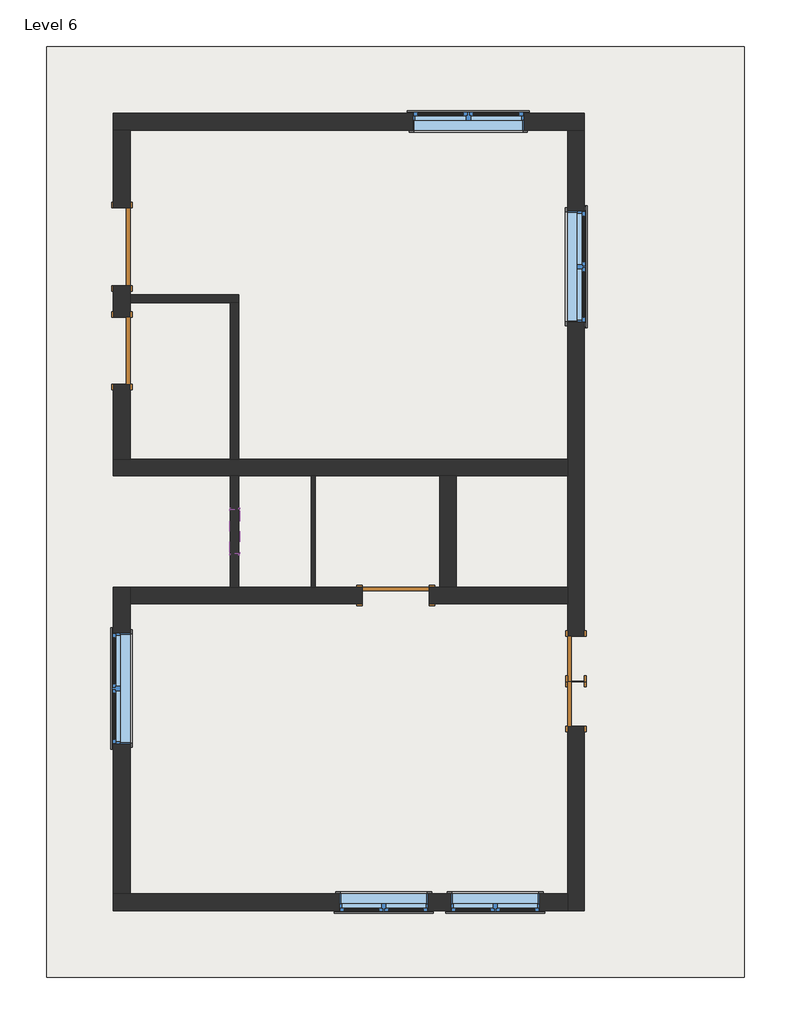
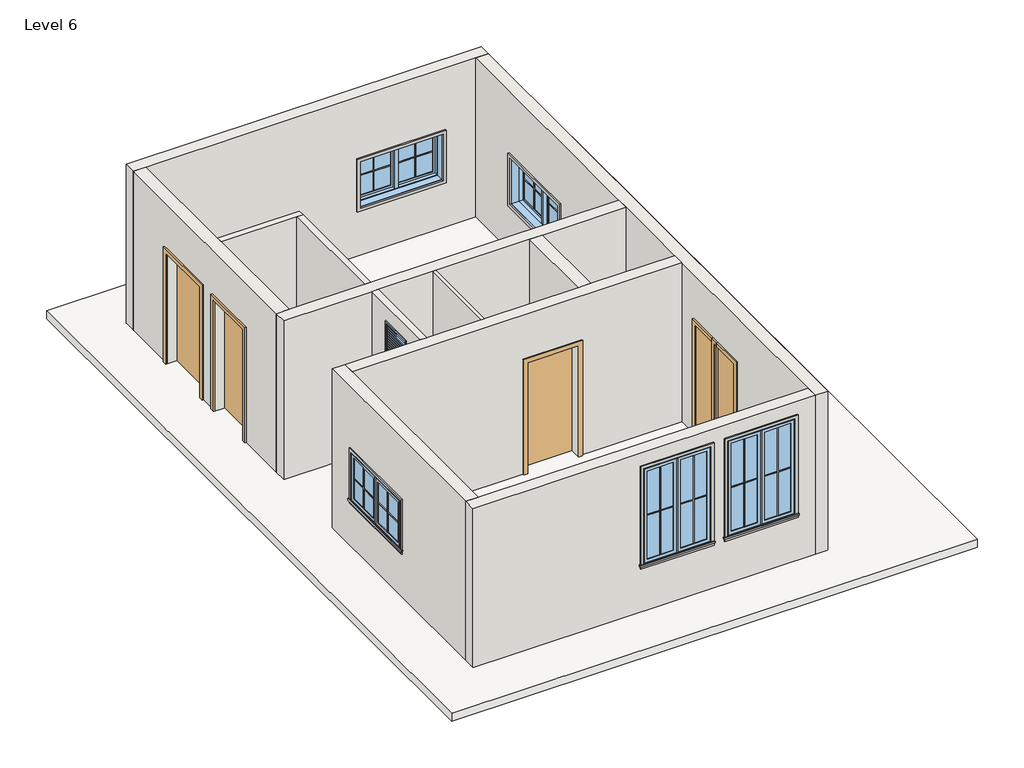
# One storey, incomplete: 20 proxies, 12 walls, 6 windows, 5 doors, 1 roof.
"""IFC4 building model written with IfcOpenShell, lengths in millimetres."""

from ifc_helpers import new_model, si_unit, frame, origin, place, context, project, spatial, polyline, outline, extrude, faceted_brep, transform, mapped, element, save
from components import muntin_pattern_2x2_muntin_pattern_2x2_9352d081, muntin_pattern_2x2_muntin_pattern_2x2_5c2cbe28, muntin_pattern_2x2_muntin_pattern_2x2_2b4d9f72, muntin_pattern_2x2_muntin_pattern_2x2_ef995ed3, trim_window_exterior_flat_with_sill_979bde60, trim_window_exterior_flat_with_sill_b7e4d11c, trim_window_interior_flat_picture_frame_7883d11b, trim_window_interior_flat_picture_frame_936b8d2a, single_flush_door_2_0d3b4037, single_flush_door_2_4a3212df, door_a90ba1ad, door_0ca8825f, door_9d399b00, window_casement_double_c1d95f0f, window_casement_double_wall_4_6ca1769e, window_d39e7ecb

model = new_model("IFC4")

# Units and contexts
model_context = context("Model", 3, world=origin())
ifc_project = project(units=[si_unit("LENGTHUNIT", "METRE", prefix="MILLI")], contexts=[model_context])

# Site, building, storey
site = spatial("IfcSite", under=ifc_project)
building = spatial("IfcBuilding", under=site)
storey = spatial("IfcBuildingStorey", under=building, Name="Level 6", Elevation=12801.6)

# Proxies
placement = place(None, origin())
muntin_pattern_2x2_muntin_pattern_2x2_shape = muntin_pattern_2x2_muntin_pattern_2x2_9352d081(model_context)
element("IfcBuildingElementProxy", 1, Name="Muntin Pattern_2x2 : Muntin Pattern_2x2", ObjectType="Muntin Pattern_2x2 : Muntin Pattern_2x2", at=placement, inside=storey, context=model_context, shape_type="MappedRepresentation", body=[
    mapped(muntin_pattern_2x2_muntin_pattern_2x2_shape, transform((-4785.3510342, -2707.8617544, 13785.85), x_axis=(0.0, 1.0, 0.0), y_axis=(-1.0, 0.0, 0.0), z_axis=(0.0, 0.0, 1.0))),
])
element("IfcBuildingElementProxy", 2, Name="Muntin Pattern_2x2 : Muntin Pattern_2x2", ObjectType="Muntin Pattern_2x2 : Muntin Pattern_2x2", at=placement, inside=storey, context=model_context, shape_type="MappedRepresentation", body=[
    mapped(muntin_pattern_2x2_muntin_pattern_2x2_shape, transform((1634.4989658, 3816.7632456, 13785.85), x_axis=(0.0, -1.0, 0.0), y_axis=(1.0, 0.0, 0.0), z_axis=(0.0, 0.0, 1.0))),
])
element("IfcBuildingElementProxy", 3, Name="Muntin Pattern_2x2 : Muntin Pattern_2x2", ObjectType="Muntin Pattern_2x2 : Muntin Pattern_2x2", at=placement, inside=storey, context=model_context, shape_type="MappedRepresentation", body=[
    mapped(muntin_pattern_2x2_muntin_pattern_2x2_shape, transform((-322.8885342, 5523.3257456, 13785.85), x_axis=(1.0, 0.0, 0.0), y_axis=(0.0, 1.0, 0.0), z_axis=(0.0, 0.0, 1.0))),
])
muntin_pattern_2x2_muntin_pattern_2x2_2_shape = muntin_pattern_2x2_muntin_pattern_2x2_5c2cbe28(model_context)
element("IfcBuildingElementProxy", 4, Name="Muntin Pattern_2x2 : Muntin Pattern_2x2", ObjectType="Muntin Pattern_2x2 : Muntin Pattern_2x2", at=placement, inside=storey, context=model_context, shape_type="MappedRepresentation", body=[
    mapped(muntin_pattern_2x2_muntin_pattern_2x2_2_shape, transform((-4785.3510342, -1949.0367544, 13785.85), x_axis=(0.0, -1.0, 0.0), y_axis=(1.0, 0.0, 0.0), z_axis=(0.0, 0.0, 1.0))),
])
element("IfcBuildingElementProxy", 5, Name="Muntin Pattern_2x2 : Muntin Pattern_2x2", ObjectType="Muntin Pattern_2x2 : Muntin Pattern_2x2", at=placement, inside=storey, context=model_context, shape_type="MappedRepresentation", body=[
    mapped(muntin_pattern_2x2_muntin_pattern_2x2_2_shape, transform((1634.4989658, 3057.9382456, 13785.85), x_axis=(0.0, 1.0, 0.0), y_axis=(-1.0, 0.0, 0.0), z_axis=(0.0, 0.0, 1.0))),
])
element("IfcBuildingElementProxy", 6, Name="Muntin Pattern_2x2 : Muntin Pattern_2x2", ObjectType="Muntin Pattern_2x2 : Muntin Pattern_2x2", at=placement, inside=storey, context=model_context, shape_type="MappedRepresentation", body=[
    mapped(muntin_pattern_2x2_muntin_pattern_2x2_2_shape, transform((435.9364658, 5523.3257456, 13785.85), x_axis=(-1.0, 0.0, 0.0), y_axis=(0.0, -1.0, 0.0), z_axis=(0.0, 0.0, 1.0))),
])
muntin_pattern_2x2_muntin_pattern_2x2_3_shape = muntin_pattern_2x2_muntin_pattern_2x2_2b4d9f72(model_context)
element("IfcBuildingElementProxy", 7, Name="Muntin Pattern_2x2 : Muntin Pattern_2x2", ObjectType="Muntin Pattern_2x2 : Muntin Pattern_2x2", at=placement, inside=storey, context=model_context, shape_type="MappedRepresentation", body=[
    mapped(muntin_pattern_2x2_muntin_pattern_2x2_3_shape, transform((-795.9635342, -5354.2242544, 13785.85), x_axis=(-1.0, 0.0, 0.0), y_axis=(0.0, -1.0, 0.0), z_axis=(0.0, 0.0, 1.0))),
])
element("IfcBuildingElementProxy", 8, Name="Muntin Pattern_2x2 : Muntin Pattern_2x2", ObjectType="Muntin Pattern_2x2 : Muntin Pattern_2x2", at=placement, inside=storey, context=model_context, shape_type="MappedRepresentation", body=[
    mapped(muntin_pattern_2x2_muntin_pattern_2x2_3_shape, transform((728.0364658, -5354.2242544, 13785.85), x_axis=(-1.0, 0.0, 0.0), y_axis=(0.0, -1.0, 0.0), z_axis=(0.0, 0.0, 1.0))),
])
muntin_pattern_2x2_muntin_pattern_2x2_4_shape = muntin_pattern_2x2_muntin_pattern_2x2_ef995ed3(model_context)
element("IfcBuildingElementProxy", 9, Name="Muntin Pattern_2x2 : Muntin Pattern_2x2", ObjectType="Muntin Pattern_2x2 : Muntin Pattern_2x2", at=placement, inside=storey, context=model_context, shape_type="MappedRepresentation", body=[
    mapped(muntin_pattern_2x2_muntin_pattern_2x2_4_shape, transform((-1402.3885342, -5354.2242544, 13785.85), x_axis=(1.0, 0.0, 0.0), y_axis=(0.0, 1.0, 0.0), z_axis=(0.0, 0.0, 1.0))),
])
element("IfcBuildingElementProxy", 10, Name="Muntin Pattern_2x2 : Muntin Pattern_2x2", ObjectType="Muntin Pattern_2x2 : Muntin Pattern_2x2", at=placement, inside=storey, context=model_context, shape_type="MappedRepresentation", body=[
    mapped(muntin_pattern_2x2_muntin_pattern_2x2_4_shape, transform((121.6114658, -5354.2242544, 13785.85), x_axis=(1.0, 0.0, 0.0), y_axis=(0.0, 1.0, 0.0), z_axis=(0.0, 0.0, 1.0))),
])
trim_window_exterior_flat_with_sill_shape = trim_window_exterior_flat_with_sill_979bde60(model_context)
element("IfcBuildingElementProxy", 11, Name="Trim-Window-Exterior-Flat : with Sill", ObjectType="Trim-Window-Exterior-Flat : with Sill", at=placement, inside=storey, context=model_context, shape_type="MappedRepresentation", body=[
    mapped(trim_window_exterior_flat_with_sill_shape, transform((-4794.8760342, -2328.4492544, 14630.4), x_axis=(0.0, -1.0, 0.0), y_axis=(0.0, 0.0, 1.0), z_axis=(-1.0, 0.0, 0.0))),
])
element("IfcBuildingElementProxy", 12, Name="Trim-Window-Exterior-Flat : with Sill", ObjectType="Trim-Window-Exterior-Flat : with Sill", at=placement, inside=storey, context=model_context, shape_type="MappedRepresentation", body=[
    mapped(trim_window_exterior_flat_with_sill_shape, transform((1644.0239658, 3437.3507456, 14630.4), x_axis=(0.0, 1.0, 0.0), y_axis=(0.0, 0.0, 1.0), z_axis=(1.0, 0.0, 0.0))),
])
element("IfcBuildingElementProxy", 13, Name="Trim-Window-Exterior-Flat : with Sill", ObjectType="Trim-Window-Exterior-Flat : with Sill", at=placement, inside=storey, context=model_context, shape_type="MappedRepresentation", body=[
    mapped(trim_window_exterior_flat_with_sill_shape, transform((56.5239658, 5532.8507456, 14630.4), x_axis=(-1.0, 0.0, 0.0), y_axis=(0.0, 0.0, 1.0), z_axis=(0.0, 1.0, 0.0))),
])
trim_window_exterior_flat_with_sill_2_shape = trim_window_exterior_flat_with_sill_b7e4d11c(model_context)
element("IfcBuildingElementProxy", 14, Name="Trim-Window-Exterior-Flat : with Sill", ObjectType="Trim-Window-Exterior-Flat : with Sill", at=placement, inside=storey, context=model_context, shape_type="MappedRepresentation", body=[
    mapped(trim_window_exterior_flat_with_sill_2_shape, transform((-1099.1760342, -5363.7492544, 15544.8), x_axis=(1.0, 0.0, 0.0), y_axis=(0.0, 0.0, 1.0), z_axis=(0.0, -1.0, 0.0))),
])
element("IfcBuildingElementProxy", 15, Name="Trim-Window-Exterior-Flat : with Sill", ObjectType="Trim-Window-Exterior-Flat : with Sill", at=placement, inside=storey, context=model_context, shape_type="MappedRepresentation", body=[
    mapped(trim_window_exterior_flat_with_sill_2_shape, transform((424.8239658, -5363.7492544, 15544.8), x_axis=(1.0, 0.0, 0.0), y_axis=(0.0, 0.0, 1.0), z_axis=(0.0, -1.0, 0.0))),
])
trim_window_interior_flat_picture_frame_shape = trim_window_interior_flat_picture_frame_7883d11b(model_context)
element("IfcBuildingElementProxy", 16, Name="Trim-Window-Interior-Flat : Picture Frame", ObjectType="Trim-Window-Interior-Flat : Picture Frame", at=placement, inside=storey, context=model_context, shape_type="MappedRepresentation", body=[
    mapped(trim_window_interior_flat_picture_frame_shape, transform((-4566.2760342, -2328.4492544, 14630.4), x_axis=(0.0, 1.0, 0.0), y_axis=(0.0, 0.0, 1.0), z_axis=(1.0, 0.0, 0.0))),
])
element("IfcBuildingElementProxy", 17, Name="Trim-Window-Interior-Flat : Picture Frame", ObjectType="Trim-Window-Interior-Flat : Picture Frame", at=placement, inside=storey, context=model_context, shape_type="MappedRepresentation", body=[
    mapped(trim_window_interior_flat_picture_frame_shape, transform((1415.4239658, 3437.3507456, 14630.4), x_axis=(0.0, -1.0, 0.0), y_axis=(0.0, 0.0, 1.0), z_axis=(-1.0, 0.0, 0.0))),
])
element("IfcBuildingElementProxy", 18, Name="Trim-Window-Interior-Flat : Picture Frame", ObjectType="Trim-Window-Interior-Flat : Picture Frame", at=placement, inside=storey, context=model_context, shape_type="MappedRepresentation", body=[
    mapped(trim_window_interior_flat_picture_frame_shape, transform((56.5239658, 5304.2507456, 14630.4), x_axis=(1.0, 0.0, 0.0), y_axis=(0.0, 0.0, 1.0), z_axis=(0.0, -1.0, 0.0))),
])
trim_window_interior_flat_picture_frame_2_shape = trim_window_interior_flat_picture_frame_936b8d2a(model_context)
element("IfcBuildingElementProxy", 19, Name="Trim-Window-Interior-Flat : Picture Frame", ObjectType="Trim-Window-Interior-Flat : Picture Frame", at=placement, inside=storey, context=model_context, shape_type="MappedRepresentation", body=[
    mapped(trim_window_interior_flat_picture_frame_2_shape, transform((-1099.1760342, -5135.1492544, 15544.8), x_axis=(-1.0, 0.0, 0.0), y_axis=(0.0, 0.0, 1.0), z_axis=(0.0, 1.0, 0.0))),
])
element("IfcBuildingElementProxy", 20, Name="Trim-Window-Interior-Flat : Picture Frame", ObjectType="Trim-Window-Interior-Flat : Picture Frame", at=placement, inside=storey, context=model_context, shape_type="MappedRepresentation", body=[
    mapped(trim_window_interior_flat_picture_frame_2_shape, transform((424.8239658, -5135.1492544, 15544.8), x_axis=(-1.0, 0.0, 0.0), y_axis=(0.0, 0.0, 1.0), z_axis=(0.0, 1.0, 0.0))),
])

# Doors
single_flush_door_2_shape = single_flush_door_2_0d3b4037(model_context)
element("IfcDoor", 21, ObjectType="Single-Flush : door 2'", at=placement, inside=storey, context=model_context, shape_type="MappedRepresentation", body=[
    mapped(single_flush_door_2_shape, transform((1529.7239658, -1922.0492544, 12801.6), x_axis=(0.0, 1.0, 0.0), y_axis=(-1.0, 0.0, 0.0), z_axis=(0.0, 0.0, 1.0))),
])
single_flush_door_2_2_shape = single_flush_door_2_4a3212df(model_context)
element("IfcDoor", 22, ObjectType="Single-Flush : door 2'", at=placement, inside=storey, context=model_context, shape_type="MappedRepresentation", body=[
    mapped(single_flush_door_2_2_shape, transform((1529.7239658, -2537.9992544, 12801.6), x_axis=(0.0, -1.0, 0.0), y_axis=(1.0, 0.0, 0.0), z_axis=(0.0, 0.0, 1.0))),
])
door_shape = door_a90ba1ad(model_context)
element("IfcDoor", 23, ObjectType="Single-Flush : door 2'6\"", at=placement, inside=storey, context=model_context, shape_type="MappedRepresentation", body=[
    mapped(door_shape, transform((-4680.5760342, 2288.0007456, 12801.6), x_axis=(0.0, 1.0, 0.0), y_axis=(-1.0, 0.0, 0.0), z_axis=(0.0, 0.0, 1.0))),
])
door_2_shape = door_0ca8825f(model_context)
element("IfcDoor", 24, ObjectType="Single-Flush : door 2'6\"", at=placement, inside=storey, context=model_context, shape_type="MappedRepresentation", body=[
    mapped(door_2_shape, transform((-934.0760342, -1058.4492544, 12801.6), x_axis=(1.0, 0.0, 0.0), y_axis=(0.0, 1.0, 0.0), z_axis=(0.0, 0.0, 1.0))),
])
door_3_shape = door_9d399b00(model_context)
element("IfcDoor", 25, ObjectType="Single-Flush : door 3'6\"", at=placement, inside=storey, context=model_context, shape_type="MappedRepresentation", body=[
    mapped(door_3_shape, transform((-4680.5760342, 3710.4007456, 12801.6), x_axis=(0.0, -1.0, 0.0), y_axis=(1.0, 0.0, 0.0), z_axis=(0.0, 0.0, 1.0))),
])

# Roof
element("IfcRoof", 26, ObjectType="roof 6\"", at=placement, inside=storey, context=model_context, shape_type="SweptSolid", body=[
    extrude(outline(polyline([(-5709.2760342, 6447.2507456), (3828.4239658, 6447.2507456), (3828.4239658, -6278.1492544), (-5709.2760342, -6278.1492544), (-5709.2760342, 6447.2507456)])), frame((0.0, 0.0, 12649.2), z_axis=(0.0, 0.0, 1.0), x_axis=(1.0, 0.0, 0.0)), (0.0, 0.0, 1.0), 152.4),
])

# Walls
element("IfcWall", 27, ObjectType="wall 2\"", at=placement, inside=storey, context=model_context, shape_type="SweptSolid", body=[
    extrude(outline(polyline([(-2089.7760342, -944.1492544), (-2089.7760342, 579.8507456), (-2038.9760342, 579.8507456), (-2038.9760342, -944.1492544), (-2089.7760342, -944.1492544)])), frame((0.0, 0.0, 12801.6), z_axis=(0.0, 0.0, 1.0), x_axis=(1.0, 0.0, 0.0)), (0.0, 0.0, 1.0), 3048.0),
])
element("IfcWall", 28, ObjectType="wall 4.5\"", at=placement, inside=storey, context=model_context, shape_type="Brep", body=[
    faceted_brep([(-4566.2760342, 2942.0507456, 12801.6), (-3194.6760342, 2942.0507456, 12801.6), (-3080.3760342, 2942.0507456, 12801.6), (-3080.3760342, 2942.0507456, 15849.6), (-3194.6760342, 2942.0507456, 15849.6), (-4566.2760342, 2942.0507456, 15849.6), (-4566.2760342, 3056.3507456, 12801.6), (-4566.2760342, 3056.3507456, 15849.6), (-3080.3760342, 3056.3507456, 15849.6), (-3080.3760342, 3056.3507456, 12801.6)], [[[0, 1, 2, 3, 4, 5]], [[6, 7, 8, 9]], [[2, 1, 0, 6, 9]], [[0, 5, 7, 6]], [[3, 2, 9, 8]], [[5, 4, 3, 8, 7]]]),
])
element("IfcWall", 29, ObjectType="wall 4.5\"", at=placement, inside=storey, context=model_context, shape_type="SweptSolid", body=[
    extrude(outline(polyline([(-3194.6760342, 808.4507456), (-3194.6760342, 2942.0507456), (-3080.3760342, 2942.0507456), (-3080.3760342, 808.4507456), (-3194.6760342, 808.4507456)])), frame((0.0, 0.0, 12801.6), z_axis=(0.0, 0.0, 1.0), x_axis=(1.0, 0.0, 0.0)), (0.0, 0.0, 1.0), 3048.0),
])
element("IfcWall", 30, ObjectType="wall 4.5\"", at=placement, inside=storey, context=model_context, shape_type="SweptSolid", body=[
    extrude(outline(polyline([(579.8507456, 12801.6), (-944.1492544, 12801.6), (-944.1492544, 15849.6), (579.8507456, 15849.6), (579.8507456, 12801.6)]), holes=[polyline([(-486.9492544, 15544.8), (-486.9492544, 14935.2), (122.6507456, 14935.2), (122.6507456, 15544.8), (-486.9492544, 15544.8)])]), frame((-3194.6760342, 0.0, 0.0), z_axis=(1.0, 0.0, 0.0), x_axis=(0.0, 1.0, 0.0)), (0.0, 0.0, 1.0), 114.3),
])
element("IfcWall", 31, ObjectType="wall 9\"", at=placement, inside=storey, context=model_context, shape_type="Brep", body=[
    faceted_brep([(-4794.8760342, 5304.2507456, 12801.6), (-4566.2760342, 5304.2507456, 12801.6), (1415.4239658, 5304.2507456, 12801.6), (1644.0239658, 5304.2507456, 12801.6), (1644.0239658, 5304.2507456, 15849.6), (1415.4239658, 5304.2507456, 15849.6), (-4566.2760342, 5304.2507456, 15849.6), (-4794.8760342, 5304.2507456, 15849.6), (818.5239658, 5304.2507456, 14630.4), (818.5239658, 5304.2507456, 13716.0), (-705.4760342, 5304.2507456, 13716.0), (-705.4760342, 5304.2507456, 14630.4), (-4794.8760342, 5532.8507456, 12801.6), (-4794.8760342, 5532.8507456, 15849.6), (1644.0239658, 5532.8507456, 15849.6), (1644.0239658, 5532.8507456, 12801.6), (818.5239658, 5532.8507456, 14630.4), (-705.4760342, 5532.8507456, 14630.4), (-705.4760342, 5532.8507456, 13716.0), (818.5239658, 5532.8507456, 13716.0)], [[[0, 1, 2, 3, 4, 5, 6, 7], [8, 9, 10, 11]], [[12, 13, 14, 15], [16, 17, 18, 19]], [[3, 2, 1, 0, 12, 15]], [[4, 3, 15, 14]], [[0, 7, 13, 12]], [[9, 8, 16, 19]], [[10, 9, 19, 18]], [[11, 10, 18, 17]], [[8, 11, 17, 16]], [[7, 6, 5, 4, 14, 13]]]),
])
element("IfcWall", 32, ObjectType="wall 9\"", at=placement, inside=storey, context=model_context, shape_type="Brep", body=[
    faceted_brep([(1415.4239658, 5304.2507456, 15849.6), (1415.4239658, 5304.2507456, 12801.6), (1415.4239658, 808.4507456, 12801.6), (1415.4239658, 579.8507456, 12801.6), (1415.4239658, -944.1492544, 12801.6), (1415.4239658, -1172.7492544, 12801.6), (1415.4239658, -1617.2492544, 12801.6), (1415.4239658, -1617.2492544, 14935.2), (1415.4239658, -2226.8492544, 14935.2), (1415.4239658, -2226.8492544, 12801.6), (1415.4239658, -2233.1992544, 12801.6), (1415.4239658, -2233.1992544, 14935.2), (1415.4239658, -2842.7992544, 14935.2), (1415.4239658, -2842.7992544, 12801.6), (1415.4239658, -5135.1492544, 12801.6), (1415.4239658, -5363.7492544, 12801.6), (1415.4239658, -5363.7492544, 15849.6), (1415.4239658, -5135.1492544, 15849.6), (1415.4239658, -1172.7492544, 15849.6), (1415.4239658, -944.1492544, 15849.6), (1415.4239658, 579.8507456, 15849.6), (1415.4239658, 808.4507456, 15849.6), (1415.4239658, 2675.3507456, 14630.4), (1415.4239658, 2675.3507456, 13716.0), (1415.4239658, 4199.3507456, 13716.0), (1415.4239658, 4199.3507456, 14630.4), (1644.0239658, 5304.2507456, 12801.6), (1644.0239658, 5304.2507456, 15849.6), (1644.0239658, -5363.7492544, 15849.6), (1644.0239658, -5363.7492544, 12801.6), (1644.0239658, -2842.7992544, 12801.6), (1644.0239658, -2842.7992544, 14935.2), (1644.0239658, -2233.1992544, 14935.2), (1644.0239658, -2233.1992544, 12801.6), (1644.0239658, -2226.8492544, 12801.6), (1644.0239658, -2226.8492544, 14935.2), (1644.0239658, -1617.2492544, 14935.2), (1644.0239658, -1617.2492544, 12801.6), (1644.0239658, 2675.3507456, 14630.4), (1644.0239658, 4199.3507456, 14630.4), (1644.0239658, 4199.3507456, 13716.0), (1644.0239658, 2675.3507456, 13716.0)], [[[0, 1, 2, 3, 4, 5, 6, 7, 8, 9, 10, 11, 12, 13, 14, 15, 16, 17, 18, 19, 20, 21], [22, 23, 24, 25]], [[26, 27, 28, 29, 30, 31, 32, 33, 34, 35, 36, 37], [38, 39, 40, 41]], [[1, 26, 37, 6, 5, 4, 3, 2]], [[29, 15, 14, 13, 30]], [[9, 34, 33, 10]], [[1, 0, 27, 26]], [[16, 15, 29, 28]], [[23, 22, 38, 41]], [[24, 23, 41, 40]], [[25, 24, 40, 39]], [[22, 25, 39, 38]], [[7, 6, 37, 36]], [[8, 7, 36, 35]], [[9, 8, 35, 34]], [[12, 31, 30, 13]], [[31, 12, 11, 32]], [[32, 11, 10, 33]], [[0, 21, 20, 19, 18, 17, 16, 28, 27]]]),
])
element("IfcWall", 33, ObjectType="wall 9\"", at=placement, inside=storey, context=model_context, shape_type="Brep", body=[
    faceted_brep([(1415.4239658, 808.4507456, 12801.6), (-3080.3760342, 808.4507456, 12801.6), (-3194.6760342, 808.4507456, 12801.6), (-4566.2760342, 808.4507456, 12801.6), (-4794.8760342, 808.4507456, 12801.6), (-4794.8760342, 808.4507456, 15849.6), (-4566.2760342, 808.4507456, 15849.6), (-3194.6760342, 808.4507456, 15849.6), (-3080.3760342, 808.4507456, 15849.6), (1415.4239658, 808.4507456, 15849.6), (1415.4239658, 579.8507456, 12801.6), (1415.4239658, 579.8507456, 15849.6), (-108.5760342, 579.8507456, 15849.6), (-337.1760342, 579.8507456, 15849.6), (-2038.9760342, 579.8507456, 15849.6), (-2089.7760342, 579.8507456, 15849.6), (-3080.3760342, 579.8507456, 15849.6), (-3194.6760342, 579.8507456, 15849.6), (-4794.8760342, 579.8507456, 15849.6), (-4794.8760342, 579.8507456, 12801.6), (-3194.6760342, 579.8507456, 12801.6), (-3080.3760342, 579.8507456, 12801.6), (-2089.7760342, 579.8507456, 12801.6), (-2038.9760342, 579.8507456, 12801.6), (-337.1760342, 579.8507456, 12801.6), (-108.5760342, 579.8507456, 12801.6)], [[[0, 1, 2, 3, 4, 5, 6, 7, 8, 9]], [[10, 11, 12, 13, 14, 15, 16, 17, 18, 19, 20, 21, 22, 23, 24, 25]], [[4, 3, 2, 1, 0, 10, 25, 24, 23, 22, 21, 20, 19]], [[0, 9, 11, 10]], [[5, 4, 19, 18]], [[9, 8, 7, 6, 5, 18, 17, 16, 15, 14, 13, 12, 11]]]),
])
element("IfcWall", 34, ObjectType="wall 9\"", at=placement, inside=storey, context=model_context, shape_type="Brep", body=[
    faceted_brep([(-4566.2760342, 2745.2007456, 14935.2), (-4566.2760342, 2745.2007456, 12801.6), (-4566.2760342, 2942.0507456, 12801.6), (-4566.2760342, 3056.3507456, 12801.6), (-4566.2760342, 3177.0007456, 12801.6), (-4566.2760342, 3177.0007456, 14935.2), (-4566.2760342, 4243.8007456, 14935.2), (-4566.2760342, 4243.8007456, 12801.6), (-4566.2760342, 5304.2507456, 12801.6), (-4566.2760342, 5304.2507456, 15849.6), (-4566.2760342, 3056.3507456, 15849.6), (-4566.2760342, 2942.0507456, 15849.6), (-4566.2760342, 808.4507456, 15849.6), (-4566.2760342, 808.4507456, 12801.6), (-4566.2760342, 1830.8007456, 12801.6), (-4566.2760342, 1830.8007456, 14935.2), (-4794.8760342, 3177.0007456, 12801.6), (-4794.8760342, 2745.2007456, 12801.6), (-4794.8760342, 2745.2007456, 14935.2), (-4794.8760342, 1830.8007456, 14935.2), (-4794.8760342, 1830.8007456, 12801.6), (-4794.8760342, 808.4507456, 12801.6), (-4794.8760342, 808.4507456, 15849.6), (-4794.8760342, 5304.2507456, 15849.6), (-4794.8760342, 5304.2507456, 12801.6), (-4794.8760342, 4243.8007456, 12801.6), (-4794.8760342, 4243.8007456, 14935.2), (-4794.8760342, 3177.0007456, 14935.2)], [[[0, 1, 2, 3, 4, 5, 6, 7, 8, 9, 10, 11, 12, 13, 14, 15]], [[16, 17, 18, 19, 20, 21, 22, 23, 24, 25, 26, 27]], [[25, 24, 8, 7]], [[14, 13, 21, 20]], [[4, 3, 2, 1, 17, 16]], [[9, 8, 24, 23]], [[13, 12, 22, 21]], [[5, 4, 16, 27]], [[6, 5, 27, 26]], [[7, 6, 26, 25]], [[18, 17, 1, 0]], [[19, 18, 0, 15]], [[20, 19, 15, 14]], [[12, 11, 10, 9, 23, 22]]]),
])
element("IfcWall", 35, ObjectType="wall 9\"", at=placement, inside=storey, context=model_context, shape_type="Brep", body=[
    faceted_brep([(1415.4239658, -5135.1492544, 12801.6), (-4566.2760342, -5135.1492544, 12801.6), (-4794.8760342, -5135.1492544, 12801.6), (-4794.8760342, -5135.1492544, 15849.6), (-4566.2760342, -5135.1492544, 15849.6), (1415.4239658, -5135.1492544, 15849.6), (-1708.7760342, -5135.1492544, 15544.8), (-1708.7760342, -5135.1492544, 13716.0), (-489.5760342, -5135.1492544, 13716.0), (-489.5760342, -5135.1492544, 15544.8), (-184.7760342, -5135.1492544, 15544.8), (-184.7760342, -5135.1492544, 13716.0), (1034.4239658, -5135.1492544, 13716.0), (1034.4239658, -5135.1492544, 15544.8), (1415.4239658, -5363.7492544, 12801.6), (1415.4239658, -5363.7492544, 15849.6), (-4794.8760342, -5363.7492544, 15849.6), (-4794.8760342, -5363.7492544, 12801.6), (-1708.7760342, -5363.7492544, 15544.8), (-489.5760342, -5363.7492544, 15544.8), (-489.5760342, -5363.7492544, 13716.0), (-1708.7760342, -5363.7492544, 13716.0), (-184.7760342, -5363.7492544, 15544.8), (1034.4239658, -5363.7492544, 15544.8), (1034.4239658, -5363.7492544, 13716.0), (-184.7760342, -5363.7492544, 13716.0)], [[[0, 1, 2, 3, 4, 5], [6, 7, 8, 9], [10, 11, 12, 13]], [[14, 15, 16, 17], [18, 19, 20, 21], [22, 23, 24, 25]], [[2, 1, 0, 14, 17]], [[0, 5, 15, 14]], [[3, 2, 17, 16]], [[7, 6, 18, 21]], [[8, 7, 21, 20]], [[9, 8, 20, 19]], [[6, 9, 19, 18]], [[11, 10, 22, 25]], [[12, 11, 25, 24]], [[13, 12, 24, 23]], [[10, 13, 23, 22]], [[5, 4, 3, 16, 15]]]),
])
element("IfcWall", 36, ObjectType="wall 9\"", at=placement, inside=storey, context=model_context, shape_type="Brep", body=[
    faceted_brep([(-4566.2760342, -5135.1492544, 12801.6), (-4566.2760342, -1172.7492544, 12801.6), (-4566.2760342, -944.1492544, 12801.6), (-4566.2760342, -944.1492544, 15849.6), (-4566.2760342, -1172.7492544, 15849.6), (-4566.2760342, -5135.1492544, 15849.6), (-4566.2760342, -1566.4492544, 14630.4), (-4566.2760342, -1566.4492544, 13716.0), (-4566.2760342, -3090.4492544, 13716.0), (-4566.2760342, -3090.4492544, 14630.4), (-4794.8760342, -5135.1492544, 12801.6), (-4794.8760342, -5135.1492544, 15849.6), (-4794.8760342, -944.1492544, 15849.6), (-4794.8760342, -944.1492544, 12801.6), (-4794.8760342, -1566.4492544, 14630.4), (-4794.8760342, -3090.4492544, 14630.4), (-4794.8760342, -3090.4492544, 13716.0), (-4794.8760342, -1566.4492544, 13716.0)], [[[0, 1, 2, 3, 4, 5], [6, 7, 8, 9]], [[10, 11, 12, 13], [14, 15, 16, 17]], [[2, 1, 0, 10, 13]], [[0, 5, 11, 10]], [[3, 2, 13, 12]], [[7, 6, 14, 17]], [[8, 7, 17, 16]], [[9, 8, 16, 15]], [[6, 9, 15, 14]], [[5, 4, 3, 12, 11]]]),
])
element("IfcWall", 37, ObjectType="wall 9\"", at=placement, inside=storey, context=model_context, shape_type="Brep", body=[
    faceted_brep([(-476.8760342, -1172.7492544, 14935.2), (-476.8760342, -1172.7492544, 12801.6), (1415.4239658, -1172.7492544, 12801.6), (1415.4239658, -1172.7492544, 15849.6), (-4566.2760342, -1172.7492544, 15849.6), (-4566.2760342, -1172.7492544, 12801.6), (-1391.2760342, -1172.7492544, 12801.6), (-1391.2760342, -1172.7492544, 14935.2), (1415.4239658, -944.1492544, 12801.6), (-108.5760342, -944.1492544, 12801.6), (-337.1760342, -944.1492544, 12801.6), (-476.8760342, -944.1492544, 12801.6), (-476.8760342, -944.1492544, 14935.2), (-1391.2760342, -944.1492544, 14935.2), (-1391.2760342, -944.1492544, 12801.6), (-2038.9760342, -944.1492544, 12801.6), (-2089.7760342, -944.1492544, 12801.6), (-3080.3760342, -944.1492544, 12801.6), (-3194.6760342, -944.1492544, 12801.6), (-4566.2760342, -944.1492544, 12801.6), (-4566.2760342, -944.1492544, 15849.6), (-3194.6760342, -944.1492544, 15849.6), (-3080.3760342, -944.1492544, 15849.6), (-2089.7760342, -944.1492544, 15849.6), (-2038.9760342, -944.1492544, 15849.6), (-337.1760342, -944.1492544, 15849.6), (-108.5760342, -944.1492544, 15849.6), (1415.4239658, -944.1492544, 15849.6)], [[[0, 1, 2, 3, 4, 5, 6, 7]], [[8, 9, 10, 11, 12, 13, 14, 15, 16, 17, 18, 19, 20, 21, 22, 23, 24, 25, 26, 27]], [[6, 5, 19, 18, 17, 16, 15, 14]], [[2, 1, 11, 10, 9, 8]], [[5, 4, 20, 19]], [[3, 2, 8, 27]], [[12, 11, 1, 0]], [[13, 12, 0, 7]], [[14, 13, 7, 6]], [[4, 3, 27, 26, 25, 24, 23, 22, 21, 20]]]),
])
element("IfcWall", 38, ObjectType="wall 9\"", at=placement, inside=storey, context=model_context, shape_type="SweptSolid", body=[
    extrude(outline(polyline([(-108.5760342, 579.8507456), (-108.5760342, -944.1492544), (-337.1760342, -944.1492544), (-337.1760342, 579.8507456), (-108.5760342, 579.8507456)])), frame((0.0, 0.0, 12801.6), z_axis=(0.0, 0.0, 1.0), x_axis=(1.0, 0.0, 0.0)), (0.0, 0.0, 1.0), 3048.0),
])

# Windows
window_casement_double_shape = window_casement_double_c1d95f0f(model_context)
element("IfcWindow", 39, ObjectType="Window-Casement-Double", at=placement, inside=storey, context=model_context, shape_type="MappedRepresentation", body=[
    mapped(window_casement_double_shape, transform((-4680.5760342, -2328.4492544, 12801.6), x_axis=(0.0, 1.0, 0.0), y_axis=(-1.0, 0.0, 0.0), z_axis=(0.0, 0.0, 1.0))),
])
element("IfcWindow", 40, ObjectType="Window-Casement-Double", at=placement, inside=storey, context=model_context, shape_type="MappedRepresentation", body=[
    mapped(window_casement_double_shape, transform((1529.7239658, 3437.3507456, 12801.6), x_axis=(0.0, -1.0, 0.0), y_axis=(1.0, 0.0, 0.0), z_axis=(0.0, 0.0, 1.0))),
])
element("IfcWindow", 41, ObjectType="Window-Casement-Double", at=placement, inside=storey, context=model_context, shape_type="MappedRepresentation", body=[
    mapped(window_casement_double_shape, transform((56.5239658, 5418.5507456, 12801.6), x_axis=(1.0, 0.0, 0.0), y_axis=(0.0, 1.0, 0.0), z_axis=(0.0, 0.0, 1.0))),
])
window_casement_double_wall_4_shape = window_casement_double_wall_4_6ca1769e(model_context)
element("IfcWindow", 42, ObjectType="Window-Casement-Double : wall 4'", at=placement, inside=storey, context=model_context, shape_type="MappedRepresentation", body=[
    mapped(window_casement_double_wall_4_shape, transform((-1099.1760342, -5249.4492544, 12801.6), x_axis=(-1.0, 0.0, 0.0), y_axis=(0.0, -1.0, 0.0), z_axis=(0.0, 0.0, 1.0))),
])
element("IfcWindow", 43, ObjectType="Window-Casement-Double : wall 4'", at=placement, inside=storey, context=model_context, shape_type="MappedRepresentation", body=[
    mapped(window_casement_double_wall_4_shape, transform((424.8239658, -5249.4492544, 12801.6), x_axis=(-1.0, 0.0, 0.0), y_axis=(0.0, -1.0, 0.0), z_axis=(0.0, 0.0, 1.0))),
])
window_shape = window_d39e7ecb(model_context)
element("IfcWindow", 44, ObjectType="Window-Louvers : 24\" x 24\"", at=placement, inside=storey, context=model_context, shape_type="MappedRepresentation", body=[
    mapped(window_shape, transform((-3143.8760342, -182.1492544, 14020.8), x_axis=(0.0, 1.0, 0.0), y_axis=(-1.0, 0.0, 0.0), z_axis=(0.0, 0.0, 1.0))),
])

save(model, "model.ifc")

# Revit data of these elements
# Type "Muntin Pattern_2x2 : Muntin Pattern_2x2"
#   Width [instance default] = 4' - 0"
#   Thickness = 0' - 0 1/2"
#   Height [instance default] = 4' - 0"
#   Distance = 0' - 0 3/4"
#   Interior Material [instance default] = none
#   Exterior Material [instance default] = none
#   Default Elevation = 0
# Type "Trim-Window-Exterior-Flat : with Sill"
#   Trim Width = 0' - 2 1/4"
#   Trim Thickness_Picture Frame = 0' - 1 1/4"
#   Trim Thickness_with Sill = 0' - 0 3/4"
#   Sill Thickness = 0' - 1 1/4"
#   Opening Width [instance default] = 2' - 0"
#   Opening Height [instance default] = 3' - 0"
#   Default Elevation = 4' - 0"
#   Sill = yes
#   Picture Frame = no
#   Trim Material [instance default] = none
# Type "Trim-Window-Interior-Flat : Picture Frame"
#   Trim Thickness_Picture Frame = 0' - 1 1/4"
#   Trim Width = 0' - 2 1/4"
#   Trim Thickness_with Sill = 0' - 0 3/4"
#   Sill Thickness = 0' - 1 1/4"
#   Opening Width [instance default] = 2' - 0"
#   Opening Height [instance default] = 3' - 0"
#   Default Elevation = 4' - 0"
#   Sill = no
#   Picture Frame = yes
#   Trim Material [instance default] = none
# Type "Single-Flush : door 2'"
#   Type Mark = "11"
#   Construction Type Id = "MDOOR"
#   Assembly Code = "C1020"
#   Analytic Construction = "Metal"
#   Thickness = 0' - 2"
#   Heat Transfer Coefficient (U) = 0.651978 BTU/(h·ft²·°F)
#   Height = 7' - 0"
#   Trim Projection Ext = 0' - 1"
#   Trim Projection Int = 0' - 1"
#   Trim Width = 0' - 3"
#   Width = 2' - 0"
#   Define Thermal Properties by = 1
#   Door Material = Door - Panel
#   Frame Material = Door - Frame
#   Visual Light Transmittance = 0
#   Solar Heat Gain Coefficient = 0
#   Function = (empty or 0)
#   Wall Closure = (empty or 0)
# Type "Single-Flush : door 2'6\""
#   Type Mark = "8"
#   Construction Type Id = "MDOOR"
#   Assembly Code = "C1020"
#   Analytic Construction = "Metal"
#   Thickness = 0' - 2"
#   Heat Transfer Coefficient (U) = 0.651978 BTU/(h·ft²·°F)
#   Height = 7' - 0"
#   Trim Projection Ext = 0' - 1"
#   Trim Projection Int = 0' - 1"
#   Trim Width = 0' - 3"
#   Width = 3' - 0"
#   Define Thermal Properties by = 1
#   Door Material = Door - Panel
#   Frame Material = Door - Frame
#   Visual Light Transmittance = 0
#   Solar Heat Gain Coefficient = 0
#   Function = (empty or 0)
#   Wall Closure = (empty or 0)
# Type "Single-Flush : door 3'6\""
#   Type Mark = "10"
#   Construction Type Id = "MDOOR"
#   Assembly Code = "C1020"
#   Analytic Construction = "Metal"
#   Thickness = 0' - 2"
#   Heat Transfer Coefficient (U) = 0.651978 BTU/(h·ft²·°F)
#   Height = 7' - 0"
#   Trim Projection Ext = 0' - 1"
#   Trim Projection Int = 0' - 1"
#   Trim Width = 0' - 3"
#   Width = 3' - 6"
#   Define Thermal Properties by = 1
#   Door Material = Door - Panel
#   Frame Material = Door - Frame
#   Visual Light Transmittance = 0
#   Solar Heat Gain Coefficient = 0
#   Function = (empty or 0)
#   Wall Closure = (empty or 0)
# Type "roof 6\""
#   Assembly Code = "B1020"
#   Layers, outside or top first: 0' - 6" no material (function 1)
# Type "wall 2\""
#   Assembly Code = "B2010"
#   Layers, outside or top first: 0' - 2" no material (function 1)
# Type "wall 4.5\""
#   Assembly Code = "B2010"
#   Layers, outside or top first: 0' - 4 1/2" no material (function 1)
# Type "wall 9\""
#   Assembly Code = "B2010"
#   Layers, outside or top first: 0' - 9" no material (function 1)
# Type "Window-Casement-Double"
#   Type Mark = "18"
#   Fire Rating = "0.5h"
#   Assembly Code = "B2020100"
#   Analytic Construction = "Double glazing - domestic"
#   Frame Extension [instance default] = 0' - 0 1/4"
#   Window Inset [instance default] = 0' - 0"
#   Wall Thickness [instance default] = 0' - 6"
#   Interior Wall Closure [instance default] = 0' - 2 1/4"
#   Half Width = 2' - 6"
#   Visual Light Transmittance = 0.81
#   Thermal Resistance (R) = 1.8146 (h·ft²·°F)/BTU
#   Solar Heat Gain Coefficient = 0.76
#   Rough Width = 5' - 0 1/2"
#   Rough Height = 3' - 0 1/2"
#   Height = 3' - 0"
#   Heat Transfer Coefficient (U) = 0.5511 BTU/(h·ft²·°F)
#   Exterior Wall Closure [instance default] = 0' - 1 1/4"
#   Extension Jamb [instance default] = 0' - 2 1/4"
#   Default Sill Height = 3' - 0"
#   Width = 5' - 0"
#   Muntin Visibility = yes
#   Interior Trim Visibility [instance default] = yes
#   Exterior Trim Visibility [instance default] = yes
#   Extension Jamb Visibility [instance default] = yes
#   Interior Trim Material = Wood - Stained
#   Muntin Pattern = Muntin Pattern_2x2 : Muntin Pattern_2x2
#   Interior Trim = Trim-Window-Interior-Flat : Picture Frame
#   Interior Frame Material = Wood - Stained
#   Glass Panel Material = Glass
#   Exterior Trim Material = Clad - White
#   Exterior Trim = Trim-Window-Exterior-Flat : with Sill
#   Exterior Frame Material = Clad - White
#   Wall Closure = (empty or 0)
# Type "Window-Casement-Double : wall 4'"
#   Type Mark = "19"
#   Fire Rating = "0.5h"
#   Assembly Code = "B2020100"
#   Analytic Construction = "Double glazing - domestic"
#   Frame Extension [instance default] = 0' - 0 1/4"
#   Window Inset [instance default] = 0' - 0"
#   Wall Thickness [instance default] = 0' - 6"
#   Interior Wall Closure [instance default] = 0' - 2 1/4"
#   Half Width = 2' - 0"
#   Visual Light Transmittance = 0.81
#   Thermal Resistance (R) = 1.8146 (h·ft²·°F)/BTU
#   Solar Heat Gain Coefficient = 0.76
#   Rough Width = 4' - 0 1/2"
#   Rough Height = 6' - 0 1/2"
#   Height = 6' - 0"
#   Heat Transfer Coefficient (U) = 0.5511 BTU/(h·ft²·°F)
#   Exterior Wall Closure [instance default] = 0' - 1 1/4"
#   Extension Jamb [instance default] = 0' - 2 1/4"
#   Default Sill Height = 3' - 0"
#   Width = 4' - 0"
#   Muntin Visibility = yes
#   Interior Trim Visibility [instance default] = yes
#   Exterior Trim Visibility [instance default] = yes
#   Extension Jamb Visibility [instance default] = yes
#   Interior Trim Material = Wood - Stained
#   Muntin Pattern = Muntin Pattern_2x2 : Muntin Pattern_2x2
#   Interior Trim = Trim-Window-Interior-Flat : Picture Frame
#   Interior Frame Material = Wood - Stained
#   Glass Panel Material = Glass
#   Exterior Trim Material = Clad - White
#   Exterior Trim = Trim-Window-Exterior-Flat : with Sill
#   Exterior Frame Material = Clad - White
#   Wall Closure = (empty or 0)
# Type "Window-Louvers : 24\" x 24\""
#   Type Mark = "20"
#   Construction Type Id = "GSP4R"
#   Assembly Code = "B20"
#   Analytic Construction = "1/8 in Pilkington single glazing"
#   Visual Light Transmittance = 0.9
#   Thermal Resistance (R) = 1.53941 (h·ft²·°F)/BTU
#   Solar Heat Gain Coefficient = 0.78
#   Max Height = 1' - 11.74264"
#   Height = 2' - 0"
#   Heat Transfer Coefficient (U) = 0.6496 BTU/(h·ft²·°F)
#   Blade Width [instance default] = 1' - 10 1/2"
#   Blade Vertical Thickness = 0' - 0.35355"
#   Blade Thickness = 0' - 0 1/4"
#   Blade Spacing = 0' - 1 1/2"
#   Blade Height = 0' - 1.85355"
#   Blade Depth = 0' - 3"
#   Blade Angle = 45.00°
#   Default Sill Height = 3' - 0"
#   Trim Projection_Exterior = 0' - 0 1/2"
#   Trim Projection_Interior = 0' - 0 1/2"
#   Trim Width_Exterior = 0' - 1 1/2"
#   Trim Width_Interior = 0' - 1 1/2"
#   Width = 2' - 0"
#   Max Blade Count = 12
#   Define Thermal Properties by = 1
#   Blade Count = 12
#   Frame Material = Birch
#   Louver Material = Birch
#   Trim Exterior Material = Birch
#   Trim Interior Material = Birch
#   Wall Closure = (empty or 0)
# Elements 1, 2, 3, 4, 5, 6 (IfcBuildingElementProxy, "Muntin Pattern_2x2 : Muntin Pattern_2x2")
#   Width = 2' - 0 5/8"
#   Height = 2' - 6 1/2"
#   Interior Material = Wood - Stained
#   Exterior Material = Clad - White
#   Phase Created = New Construction
#   Materials on its faces: "Clad - White", "Wood - Stained"
# Elements 7, 8, 9, 10 (IfcBuildingElementProxy, "Muntin Pattern_2x2 : Muntin Pattern_2x2")
#   Width = 1' - 6 5/8"
#   Height = 5' - 6 1/2"
#   Interior Material = Wood - Stained
#   Exterior Material = Clad - White
#   Phase Created = New Construction
#   Materials on its faces: "Clad - White", "Wood - Stained"
# Elements 11, 12, 13 (IfcBuildingElementProxy, "Trim-Window-Exterior-Flat : with Sill")
#   Opening Width = 5' - 0"
#   Opening Height = 3' - 0"
#   Trim Material = Clad - White
#   Phase Created = New Construction
#   Materials on its faces: "Clad - White"
# Elements 14, 15 (IfcBuildingElementProxy, "Trim-Window-Exterior-Flat : with Sill")
#   Opening Width = 4' - 0"
#   Opening Height = 6' - 0"
#   Trim Material = Clad - White
#   Phase Created = New Construction
#   Materials on its faces: "Clad - White"
# Elements 16, 17, 18 (IfcBuildingElementProxy, "Trim-Window-Interior-Flat : Picture Frame")
#   Opening Width = 5' - 0"
#   Opening Height = 3' - 0"
#   Trim Material = Wood - Stained
#   Phase Created = New Construction
#   Materials on its faces: "Wood - Stained"
# Elements 19, 20 (IfcBuildingElementProxy, "Trim-Window-Interior-Flat : Picture Frame")
#   Opening Width = 4' - 0"
#   Opening Height = 6' - 0"
#   Trim Material = Wood - Stained
#   Phase Created = New Construction
#   Materials on its faces: "Wood - Stained"
# Elements 21, 22 (IfcDoor, "Single-Flush : door 2'")
#   Phase Created = New Construction
#   Materials on its faces: "Door - Frame", "Door - Panel"
# Elements 23, 24 (IfcDoor, "Single-Flush : door 2'6\"")
#   Phase Created = New Construction
#   Materials on its faces: "Door - Frame", "Door - Panel"
# Element 25 (IfcDoor, "Single-Flush : door 3'6\"")
#   Phase Created = New Construction
#   Materials on its faces: "Door - Frame", "Door - Panel"
# Element 26 (IfcRoof, "roof 6\"")
#   built-in parameter 1001705 = 42 (stored number, unit not read)
#   built-in parameter 1001701 = -0.5 (stored number, unit not read)
#   built-in parameter 1001710 = 33615
#   Phase Created = New Construction
#   Materials on its faces: "Copper", "Default Roof", "Wood - Stained"
# Element 27 (IfcWall, "wall 2\"")
#   Top Offset = 0' - 0"
#   Base Offset = 0' - 0"
#   Unconnected Height = 10' - 0"
#   wall height = 10' - 0"
#   Phase Created = New Construction
#   Base Constraint = Level 6
#   Materials on its faces: "Default Wall"
# Elements 28, 29 (IfcWall, "wall 4.5\"")
#   Top Offset = 0' - 0"
#   Base Offset = 0' - 0"
#   Unconnected Height = 10' - 0"
#   wall height = 10' - 0"
#   Phase Created = New Construction
#   Base Constraint = Level 6
#   Materials on its faces: "Default Wall"
# Element 30 (IfcWall, "wall 4.5\"")
#   Top Offset = 0' - 0"
#   Base Offset = 0' - 0"
#   Unconnected Height = 10' - 0"
#   wall height = 10' - 0"
#   Phase Created = New Construction
#   Base Constraint = Level 6
#   Materials on its faces: "Default Wall", "Wood Planks"
# Elements 31, 32, 33, 35, 36, 37 (IfcWall, "wall 9\"")
#   Top Offset = 0' - 0"
#   Base Offset = 0' - 0"
#   Unconnected Height = 10' - 0"
#   wall height = 10' - 0"
#   Phase Created = New Construction
#   Base Constraint = Level 6
#   Materials on its faces: "Default Wall", "Wood Planks"
# Element 34 (IfcWall, "wall 9\"")
#   Top Offset = 0' - 0"
#   Base Offset = 0' - 0"
#   Unconnected Height = 10' - 0"
#   wall height = 10' - 0"
#   Phase Created = New Construction
#   Base Constraint = Level 6
#   Materials on its faces: "Default Wall", "Copper", "Wood Planks"
# Element 38 (IfcWall, "wall 9\"")
#   Top Offset = 0' - 0"
#   Base Offset = 0' - 0"
#   Unconnected Height = 10' - 0"
#   wall height = 10' - 0"
#   Phase Created = New Construction
#   Base Constraint = Level 6
#   Materials on its faces: "Default Wall"
# Element 39 (IfcWindow, "Window-Casement-Double")
#   Mark = "25"
#   Window Inset = 0' - 0"
#   Interior Wall Closure = 0' - 2 1/4"
#   Frame Extension = 0' - 0 1/4"
#   Exterior Wall Closure = 0' - 1 1/4"
#   Interior Trim Visibility = yes
#   Exterior Trim Visibility = yes
#   Phase Created = New Construction
#   Materials on its faces: "Wood - Stained", "Glass", "Clad - White"
# Element 40 (IfcWindow, "Window-Casement-Double")
#   Mark = "26"
#   Window Inset = 0' - 0"
#   Interior Wall Closure = 0' - 2 1/4"
#   Frame Extension = 0' - 0 1/4"
#   Exterior Wall Closure = 0' - 1 1/4"
#   Interior Trim Visibility = yes
#   Exterior Trim Visibility = yes
#   Phase Created = New Construction
#   Materials on its faces: "Wood - Stained", "Glass", "Clad - White"
# Element 41 (IfcWindow, "Window-Casement-Double")
#   Mark = "27"
#   Window Inset = 0' - 0"
#   Interior Wall Closure = 0' - 2 1/4"
#   Frame Extension = 0' - 0 1/4"
#   Exterior Wall Closure = 0' - 1 1/4"
#   Interior Trim Visibility = yes
#   Exterior Trim Visibility = yes
#   Phase Created = New Construction
#   Materials on its faces: "Wood - Stained", "Glass", "Clad - White"
# Element 42 (IfcWindow, "Window-Casement-Double : wall 4'")
#   Mark = "28"
#   Window Inset = 0' - 0"
#   Interior Wall Closure = 0' - 2 1/4"
#   Frame Extension = 0' - 0 1/4"
#   Exterior Wall Closure = 0' - 1 1/4"
#   Interior Trim Visibility = yes
#   Exterior Trim Visibility = yes
#   Phase Created = New Construction
#   Materials on its faces: "Wood - Stained", "Glass", "Clad - White"
# Element 43 (IfcWindow, "Window-Casement-Double : wall 4'")
#   Mark = "29"
#   Window Inset = 0' - 0"
#   Interior Wall Closure = 0' - 2 1/4"
#   Frame Extension = 0' - 0 1/4"
#   Exterior Wall Closure = 0' - 1 1/4"
#   Interior Trim Visibility = yes
#   Exterior Trim Visibility = yes
#   Phase Created = New Construction
#   Materials on its faces: "Wood - Stained", "Glass", "Clad - White"
# Element 44 (IfcWindow, "Window-Louvers : 24\" x 24\"")
#   Mark = "30"
#   Blade Width = 1' - 10 1/2"
#   Phase Created = New Construction
#   Materials on its faces: "Birch"
# Materials
#   "Door - Panel": class "Wood", colour RGB 210 159 95, transparency 0, Cost = 0
#   "Door - Frame": colour RGB 118 70 51, transparency 0, Cost = 0
#   "Wood - Stained": class "Wood", colour RGB 224 178 126, transparency 0, Cost = 0
#   "Glass": class "Glass", colour RGB 0 128 192, transparency 0.75, Description = "Soda Lime Glass", Cost = 0
#   "Clad - White": class "Wood", colour RGB 242 242 238, transparency 0, Cost = 0
#   "Birch": class "Wood", colour RGB 224 178 126, transparency 0, Description = "Betula Alleghaniensis", Cost = 0
#   "Copper": class "Metal", colour RGB 0 0 0, transparency 0, Description = "Copper, matte finish", Cost = 0
#   "Default Roof": colour RGB 88 101 114, transparency 0, Cost = 0
#   "Default Wall": colour RGB 128 128 128, transparency 0, Cost = 0
#   "Wood Planks": class "Wood", colour RGB 193 160 115, transparency 0, Description = "Physical material.", Cost = 0
